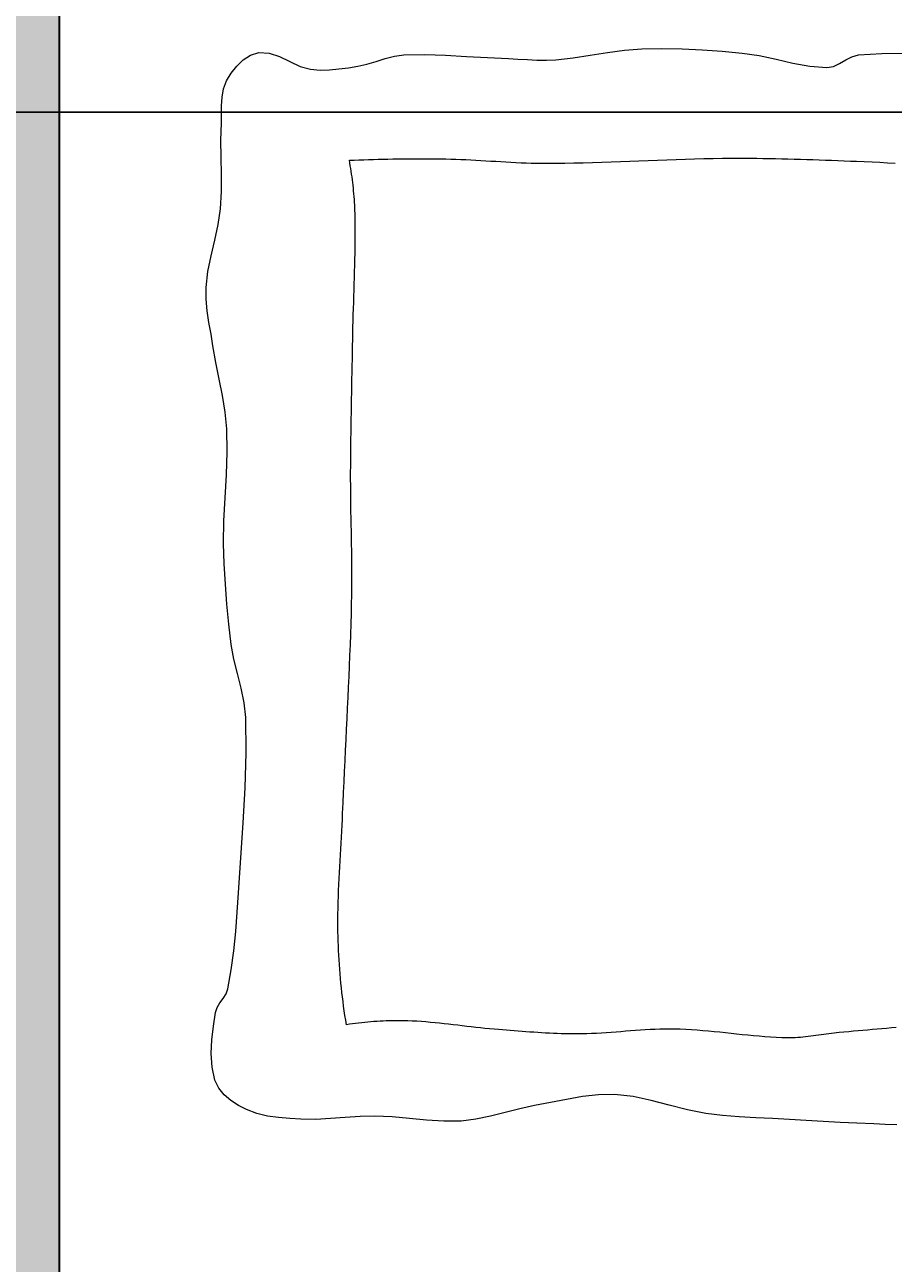
# Model space of a CAD drawing. Units: inches. Extents: x -15 to 423, y -713 to 71.
# Tile 11 of 24: x 251 to 308, y -351 to -270. Entities that reach past the tile are written whole.
import ezdxf

# ---------------------------------------------------------------- set-up
doc = ezdxf.new("R2010")
doc.units = ezdxf.units.IN
doc.header["$MEASUREMENT"] = 0
for name, color, linetype, lineweight in [('A-ANNO-DIMS', 2, 'Continuous', 18), ('A-FURN', 9, 'Continuous', 13), ('A-WALL', 7, 'Continuous', 35), ('A-WALL-PATT', 8, 'Continuous', 13)]:
    doc.layers.add(name, color=color, linetype=linetype, lineweight=lineweight)
doc.styles.get("Standard").update_dxf_attribs({"font": 'arial.ttf'})
doc.dimstyles.get("Standard").update_dxf_attribs({"dimtxt": 0.18, "dimasz": 0.18, "dimexe": 0.18, "dimexo": 0.0625, "dimgap": 0.09, "dimtad": 0, "dimtih": 1, "dimtoh": 1, "dimdec": 0, "dimzin": 0, "dimdsep": 46, "dimlunit": 3, "dimtxsty": 'Standard', "dimcen": 0.09, "dimadec": 0, "dimazin": 0, "dimtfac": 1, "dimtdec": 0, "dimtofl": 0, "dimtmove": 0, "dimatfit": 3, "dimfxl": 1, "dimtolj": 1, "dimtzin": 0, "dimarcsym": 0})

# ---------------------------------------------------------------- blocks, each defined once
blk = doc.blocks.new('BED-DOUBLE')
for p, q in [((2.003, 69.219), (2.429, 69.63)), ((2.429, 69.63), (2.912, 69.937)), ((2.912, 69.937), (3.444, 70.1)), ((3.444, 70.1), (4.136, 70.064)), ((4.136, 70.064), (4.809, 69.832)), ((4.809, 69.832), (5.474, 69.509)), ((11.118, 69.518), (11.713, 69.708)), ((11.713, 69.708), (12.313, 69.864)), ((12.313, 69.864), (12.925, 69.947)), ((12.925, 69.947), (14.291, 69.973)), ((14.291, 69.973), (15.658, 69.932)), ((15.658, 69.932), (17.025, 69.853)), ((17.025, 69.853), (18.393, 69.767)), ((18.393, 69.767), (19.76, 69.702)), ((19.76, 69.702), (20.382, 69.674)), ((20.382, 69.674), (21.004, 69.639)), ((21.004, 69.639), (21.626, 69.611)), ((21.626, 69.611), (22.247, 69.602)), ((22.247, 69.602), (22.868, 69.627)), ((22.868, 69.627), (23.993, 69.748)), ((23.993, 69.748), (25.114, 69.92)), ((25.114, 69.92), (26.233, 70.103)), ((26.233, 70.103), (27.355, 70.258)), ((27.355, 70.258), (28.482, 70.345)), ((28.482, 70.345), (29.796, 70.368)), ((29.796, 70.368), (31.11, 70.346)), ((31.11, 70.346), (32.424, 70.284)), ((32.424, 70.284), (33.736, 70.19)), ((33.736, 70.19), (35.045, 70.069)), ((35.045, 70.069), (36.156, 69.9)), ((36.156, 69.9), (37.259, 69.661)), ((37.259, 69.661), (38.359, 69.412)), ((41.413, 69.382), (41.81, 69.617)), ((41.81, 69.617), (42.214, 69.827)), ((42.214, 69.827), (42.641, 69.942)), ((42.641, 69.942), (44.16, 70.042)), ((44.16, 70.042), (45.684, 70.067)), ((1.638, 68.744), (2.003, 69.219)), ((5.474, 69.509), (6.146, 69.198)), ((6.146, 69.198), (6.838, 69.007)), ((6.838, 69.007), (7.451, 68.958)), ((7.451, 68.958), (8.068, 68.97)), ((8.068, 68.97), (8.686, 69.026)), ((8.686, 69.026), (9.302, 69.109)), ((9.302, 69.109), (9.914, 69.204)), ((9.914, 69.204), (10.52, 69.337)), ((10.52, 69.337), (11.118, 69.518)), ((38.359, 69.412), (39.464, 69.211)), ((39.464, 69.211), (40.58, 69.118)), ((40.58, 69.118), (41.008, 69.192)), ((41.008, 69.192), (41.413, 69.382)), ((1.142, 67.735), (1.339, 68.246)), ((1.339, 68.246), (1.638, 68.744)), ((1.014, 66.627), (1.045, 67.191)), ((1.045, 67.191), (1.142, 67.735)), ((1.011, 66.057), (1.014, 66.627)), ((1, 65.495), (1.011, 66.057)), ((0.976, 64.376), (1, 65.495)), ((0.991, 63.255), (0.976, 64.376)), ((1.011, 62.135), (0.991, 63.255)), ((10.94, 63.119), (11.255, 63.127)), ((11.255, 63.127), (11.57, 63.134)), ((11.57, 63.134), (11.885, 63.14)), ((11.885, 63.14), (12.2, 63.145)), ((12.2, 63.145), (12.515, 63.15)), ((12.515, 63.15), (12.83, 63.153)), ((12.83, 63.153), (13.145, 63.156)), ((13.145, 63.156), (13.46, 63.158)), ((13.46, 63.158), (13.775, 63.159)), ((13.775, 63.159), (14.09, 63.159)), ((14.09, 63.159), (14.405, 63.158)), ((14.405, 63.158), (14.72, 63.156)), ((14.72, 63.156), (15.035, 63.154)), ((15.035, 63.154), (15.35, 63.15)), ((15.35, 63.15), (15.665, 63.146)), ((15.665, 63.146), (15.993, 63.139)), ((15.993, 63.139), (16.321, 63.13)), ((16.321, 63.13), (16.649, 63.118)), ((30.721, 63.116), (31.328, 63.135)), ((31.328, 63.135), (31.935, 63.153)), ((31.935, 63.153), (32.542, 63.168)), ((32.542, 63.168), (33.148, 63.181)), ((33.148, 63.181), (33.755, 63.19)), ((33.755, 63.19), (34.362, 63.196)), ((34.362, 63.196), (34.77, 63.197)), ((34.77, 63.197), (35.178, 63.197)), ((35.178, 63.197), (35.586, 63.195)), ((35.586, 63.195), (35.994, 63.192)), ((35.994, 63.192), (36.402, 63.187)), ((36.402, 63.187), (36.81, 63.18)), ((36.81, 63.18), (37.218, 63.172)), ((37.218, 63.172), (37.626, 63.163)), ((37.626, 63.163), (38.034, 63.153)), ((38.034, 63.153), (38.442, 63.142)), ((38.442, 63.142), (38.85, 63.13)), ((38.85, 63.13), (39.258, 63.117)), ((9.366, 63.066), (9.681, 63.078)), ((9.399, 62.885), (9.366, 63.066)), ((9.431, 62.703), (9.399, 62.885)), ((9.461, 62.522), (9.431, 62.703)), ((9.49, 62.34), (9.461, 62.522)), ((9.518, 62.157), (9.49, 62.34)), ((9.681, 63.078), (9.995, 63.09)), ((9.995, 63.09), (10.31, 63.1)), ((10.31, 63.1), (10.625, 63.11)), ((10.625, 63.11), (10.94, 63.119)), ((16.649, 63.118), (16.978, 63.104)), ((16.978, 63.104), (17.306, 63.088)), ((17.306, 63.088), (17.634, 63.07)), ((17.634, 63.07), (17.962, 63.052)), ((17.962, 63.052), (18.29, 63.032)), ((18.29, 63.032), (18.618, 63.013)), ((18.618, 63.013), (18.946, 62.993)), ((18.946, 62.993), (19.274, 62.973)), ((19.274, 62.973), (19.602, 62.954)), ((19.602, 62.954), (19.93, 62.937)), ((19.93, 62.937), (20.258, 62.92)), ((20.258, 62.92), (20.586, 62.905)), ((20.586, 62.905), (20.914, 62.893)), ((20.914, 62.893), (21.242, 62.882)), ((21.242, 62.882), (21.57, 62.875)), ((21.57, 62.875), (21.899, 62.87)), ((21.899, 62.87), (22.227, 62.869)), ((22.227, 62.869), (22.834, 62.873)), ((22.834, 62.873), (23.441, 62.88)), ((23.441, 62.88), (24.048, 62.891)), ((24.048, 62.891), (24.654, 62.905)), ((24.654, 62.905), (25.261, 62.921)), ((25.261, 62.921), (25.868, 62.94)), ((25.868, 62.94), (26.475, 62.96)), ((26.475, 62.96), (27.081, 62.982)), ((27.081, 62.982), (27.688, 63.004)), ((27.688, 63.004), (28.295, 63.027)), ((28.295, 63.027), (28.901, 63.05)), ((28.901, 63.05), (29.508, 63.073)), ((29.508, 63.073), (30.115, 63.095)), ((30.115, 63.095), (30.721, 63.116)), ((39.258, 63.117), (39.666, 63.103)), ((39.666, 63.103), (40.073, 63.089)), ((40.073, 63.089), (40.481, 63.074)), ((40.481, 63.074), (40.889, 63.059)), ((40.889, 63.059), (41.297, 63.044)), ((41.297, 63.044), (41.705, 63.028)), ((41.705, 63.028), (42.112, 63.013)), ((42.112, 63.013), (42.52, 62.997)), ((42.52, 62.997), (43.024, 62.977)), ((43.024, 62.977), (43.528, 62.954)), ((43.528, 62.954), (44.032, 62.93)), ((44.032, 62.93), (44.535, 62.904)), ((44.535, 62.904), (45.039, 62.877)), ((1.006, 61.015), (1.011, 62.135)), ((9.543, 61.975), (9.518, 62.157)), ((9.568, 61.792), (9.543, 61.975)), ((9.59, 61.609), (9.568, 61.792)), ((9.612, 61.426), (9.59, 61.609)), ((0.942, 59.899), (1.006, 61.015)), ((9.631, 61.242), (9.612, 61.426)), ((9.649, 61.059), (9.631, 61.242)), ((9.666, 60.875), (9.649, 61.059)), ((9.681, 60.691), (9.666, 60.875)), ((0.791, 58.864), (0.942, 59.899)), ((9.694, 60.507), (9.681, 60.691)), ((9.706, 60.323), (9.694, 60.507)), ((9.717, 60.139), (9.706, 60.323)), ((9.726, 59.955), (9.717, 60.139)), ((9.733, 59.771), (9.726, 59.955)), ((9.739, 59.587), (9.733, 59.771)), ((9.743, 59.403), (9.739, 59.587)), ((9.749, 59.001), (9.743, 59.403)), ((0.568, 57.839), (0.791, 58.864)), ((9.752, 58.599), (9.749, 59.001)), ((9.753, 58.197), (9.752, 58.599)), ((0.326, 56.816), (0.568, 57.839)), ((9.746, 57.392), (9.751, 57.794)), ((9.751, 57.794), (9.753, 58.197)), ((0.119, 55.79), (0.326, 56.816)), ((9.732, 56.588), (9.74, 56.99)), ((9.74, 56.99), (9.746, 57.392)), ((9.713, 55.784), (9.723, 56.186)), ((9.723, 56.186), (9.732, 56.588)), ((0, 54.752), (0.119, 55.79)), ((9.689, 54.98), (9.701, 55.382)), ((9.701, 55.382), (9.713, 55.784)), ((0.002, 53.985), (0, 54.752)), ((9.663, 54.176), (9.676, 54.578)), ((9.676, 54.578), (9.689, 54.98)), ((0.074, 53.22), (0.002, 53.985)), ((9.637, 53.371), (9.65, 53.773)), ((9.65, 53.773), (9.663, 54.176)), ((0.191, 52.456), (0.074, 53.22)), ((9.614, 52.567), (9.625, 52.969)), ((9.625, 52.969), (9.637, 53.371)), ((0.325, 51.694), (0.191, 52.456)), ((9.594, 51.763), (9.603, 52.165)), ((9.603, 52.165), (9.614, 52.567)), ((0.451, 50.932), (0.325, 51.694)), ((9.579, 50.926), (9.586, 51.361)), ((9.586, 51.361), (9.594, 51.763)), ((0.64, 49.847), (0.451, 50.932)), ((9.562, 50.055), (9.571, 50.49)), ((9.571, 50.49), (9.579, 50.926)), ((0.862, 48.766), (0.64, 49.847)), ((9.546, 49.185), (9.554, 49.62)), ((9.554, 49.62), (9.562, 50.055)), ((1.08, 47.685), (0.862, 48.766)), ((9.529, 48.315), (9.537, 48.75)), ((9.537, 48.75), (9.546, 49.185)), ((9.512, 47.444), (9.521, 47.879)), ((9.521, 47.879), (9.529, 48.315)), ((1.261, 46.6), (1.08, 47.685)), ((9.497, 46.574), (9.505, 47.009)), ((9.505, 47.009), (9.512, 47.444)), ((1.369, 45.507), (1.261, 46.6)), ((9.483, 45.704), (9.49, 46.139)), ((9.49, 46.139), (9.497, 46.574)), ((1.392, 44.009), (1.369, 45.507)), ((9.477, 45.268), (9.483, 45.704)), ((9.466, 44.398), (9.471, 44.833)), ((9.471, 44.833), (9.477, 45.268)), ((1.334, 42.51), (1.392, 44.009)), ((9.457, 43.528), (9.461, 43.963)), ((9.461, 43.963), (9.466, 44.398)), ((9.452, 42.657), (9.454, 43.092)), ((9.454, 43.092), (9.457, 43.528)), ((1.242, 41.01), (1.334, 42.51)), ((9.451, 42.232), (9.452, 42.657)), ((9.453, 41.806), (9.451, 42.232)), ((9.456, 41.38), (9.453, 41.806)), ((9.461, 40.954), (9.456, 41.38)), ((1.164, 39.51), (1.242, 41.01)), ((9.467, 40.529), (9.461, 40.954)), ((9.474, 40.103), (9.467, 40.529)), ((9.481, 39.677), (9.474, 40.103)), ((9.489, 39.251), (9.481, 39.677)), ((1.147, 38.01), (1.164, 39.51)), ((9.497, 38.826), (9.489, 39.251)), ((9.505, 38.4), (9.497, 38.826)), ((9.513, 37.974), (9.505, 38.4)), ((1.189, 36.691), (1.147, 38.01)), ((9.519, 37.548), (9.513, 37.974)), ((9.525, 37.123), (9.519, 37.548)), ((1.262, 35.372), (1.189, 36.691)), ((9.53, 36.697), (9.525, 37.123)), ((9.533, 36.271), (9.53, 36.697)), ((9.535, 35.846), (9.533, 36.271)), ((9.534, 35.42), (9.535, 35.846)), ((1.364, 34.055), (1.262, 35.372)), ((9.525, 34.569), (9.531, 34.994)), ((9.531, 34.994), (9.534, 35.42)), ((1.493, 32.741), (1.364, 34.055)), ((9.499, 33.455), (9.517, 34.143)), ((9.517, 34.143), (9.525, 34.569)), ((9.479, 32.766), (9.499, 33.455)), ((1.648, 31.429), (1.493, 32.741)), ((9.457, 32.078), (9.479, 32.766)), ((9.433, 31.389), (9.457, 32.078)), ((1.821, 30.468), (1.648, 31.429)), ((9.406, 30.701), (9.433, 31.389)), ((2.058, 29.516), (1.821, 30.468)), ((9.349, 29.324), (9.378, 30.012)), ((9.378, 30.012), (9.406, 30.701)), ((2.303, 28.566), (2.058, 29.516)), ((9.318, 28.636), (9.349, 29.324)), ((2.502, 27.612), (2.303, 28.566)), ((9.286, 27.948), (9.318, 28.636)), ((2.6, 26.645), (2.502, 27.612)), ((9.254, 27.26), (9.286, 27.948)), ((9.221, 26.572), (9.254, 27.26)), ((2.618, 24.352), (2.6, 26.645)), ((9.187, 25.883), (9.221, 26.572)), ((9.12, 24.507), (9.153, 25.195)), ((9.153, 25.195), (9.187, 25.883)), ((2.555, 22.06), (2.618, 24.352)), ((9.086, 23.819), (9.12, 24.507)), ((9.053, 23.131), (9.086, 23.819)), ((9.02, 22.443), (9.053, 23.131)), ((2.435, 19.769), (2.555, 22.06)), ((8.989, 21.755), (9.02, 22.443)), ((8.929, 20.378), (8.958, 21.066)), ((8.958, 21.066), (8.989, 21.755)), ((8.912, 19.992), (8.929, 20.378)), ((2.283, 17.478), (2.435, 19.769)), ((8.873, 19.219), (8.893, 19.606)), ((8.893, 19.606), (8.912, 19.992)), ((8.83, 18.447), (8.852, 18.833)), ((8.852, 18.833), (8.873, 19.219)), ((8.785, 17.674), (8.807, 18.06)), ((8.807, 18.06), (8.83, 18.447)), ((2.127, 15.19), (2.283, 17.478)), ((8.74, 16.901), (8.762, 17.288)), ((8.762, 17.288), (8.785, 17.674)), ((8.699, 16.129), (8.719, 16.515)), ((8.719, 16.515), (8.74, 16.901)), ((8.664, 15.356), (8.681, 15.742)), ((8.681, 15.742), (8.699, 16.129)), ((2.039, 13.928), (2.127, 15.19)), ((8.628, 14.197), (8.637, 14.583)), ((8.637, 14.583), (8.649, 14.97)), ((8.649, 14.97), (8.664, 15.356)), ((1.937, 12.667), (2.039, 13.928)), ((8.619, 13.424), (8.622, 13.81)), ((8.622, 13.81), (8.628, 14.197)), ((8.619, 13.037), (8.619, 13.424)), ((8.624, 12.651), (8.619, 13.037)), ((1.808, 11.408), (1.937, 12.667)), ((8.631, 12.346), (8.624, 12.651)), ((8.64, 12.04), (8.631, 12.346)), ((1.642, 10.155), (1.808, 11.408)), ((8.651, 11.735), (8.64, 12.04)), ((8.664, 11.43), (8.651, 11.735)), ((8.679, 11.125), (8.664, 11.43)), ((8.697, 10.82), (8.679, 11.125)), ((8.717, 10.516), (8.697, 10.82)), ((1.43, 8.91), (1.642, 10.155)), ((8.739, 10.211), (8.717, 10.516)), ((8.763, 9.906), (8.739, 10.211)), ((8.79, 9.602), (8.763, 9.906)), ((1.31, 8.587), (1.43, 8.91)), ((8.818, 9.298), (8.79, 9.602)), ((8.849, 8.994), (8.818, 9.298)), ((8.883, 8.69), (8.849, 8.994)), ((0.905, 7.999), (1.119, 8.289)), ((1.119, 8.289), (1.31, 8.587)), ((8.918, 8.387), (8.883, 8.69)), ((8.955, 8.084), (8.918, 8.387)), ((0.489, 6.488), (0.615, 7.375)), ((0.615, 7.375), (0.72, 7.7)), ((0.72, 7.7), (0.905, 7.999)), ((8.995, 7.781), (8.955, 8.084)), ((9.037, 7.479), (8.995, 7.781)), ((9.081, 7.176), (9.037, 7.479)), ((0.386, 5.589), (0.489, 6.488)), ((9.127, 6.875), (9.081, 7.176)), ((9.176, 6.573), (9.127, 6.875)), ((9.374, 6.604), (9.176, 6.573)), ((9.573, 6.633), (9.374, 6.604)), ((9.773, 6.66), (9.573, 6.633)), ((9.972, 6.685), (9.773, 6.66)), ((10.172, 6.708), (9.972, 6.685)), ((10.372, 6.729), (10.172, 6.708)), ((10.573, 6.748), (10.372, 6.729)), ((10.773, 6.766), (10.573, 6.748)), ((10.974, 6.781), (10.773, 6.766)), ((11.175, 6.795), (10.974, 6.781)), ((11.376, 6.806), (11.175, 6.795)), ((11.577, 6.816), (11.376, 6.806)), ((11.778, 6.824), (11.577, 6.816)), ((11.979, 6.83), (11.778, 6.824)), ((12.18, 6.834), (11.979, 6.83)), ((12.382, 6.836), (12.18, 6.834)), ((12.583, 6.836), (12.382, 6.836)), ((12.784, 6.835), (12.583, 6.836)), ((12.985, 6.831), (12.784, 6.835)), ((13.186, 6.826), (12.985, 6.831)), ((13.483, 6.814), (13.186, 6.826)), ((13.781, 6.798), (13.483, 6.814)), ((14.078, 6.779), (13.781, 6.798)), ((14.375, 6.756), (14.078, 6.779)), ((14.672, 6.731), (14.375, 6.756)), ((14.969, 6.703), (14.672, 6.731)), ((15.265, 6.673), (14.969, 6.703)), ((15.561, 6.641), (15.265, 6.673)), ((15.858, 6.607), (15.561, 6.641)), ((16.154, 6.573), (15.858, 6.607)), ((16.45, 6.538), (16.154, 6.573)), ((16.746, 6.503), (16.45, 6.538)), ((17.043, 6.467), (16.746, 6.503)), ((17.339, 6.432), (17.043, 6.467)), ((17.635, 6.398), (17.339, 6.432)), ((17.932, 6.366), (17.635, 6.398)), ((18.228, 6.334), (17.932, 6.366)), ((18.525, 6.305), (18.228, 6.334)), ((18.822, 6.278), (18.525, 6.305)), ((19.119, 6.254), (18.822, 6.278)), ((19.375, 6.234), (19.119, 6.254)), ((19.63, 6.214), (19.375, 6.234)), ((19.886, 6.194), (19.63, 6.214)), ((20.142, 6.174), (19.886, 6.194)), ((20.398, 6.154), (20.142, 6.174)), ((20.654, 6.134), (20.398, 6.154)), ((20.91, 6.115), (20.654, 6.134)), ((21.166, 6.097), (20.91, 6.115)), ((21.423, 6.079), (21.166, 6.097)), ((21.679, 6.062), (21.423, 6.079)), ((21.935, 6.047), (21.679, 6.062)), ((22.191, 6.032), (21.935, 6.047)), ((22.448, 6.019), (22.191, 6.032)), ((22.704, 6.007), (22.448, 6.019)), ((22.96, 5.997), (22.704, 6.007)), ((23.217, 5.988), (22.96, 5.997)), ((23.473, 5.981), (23.217, 5.988)), ((23.73, 5.977), (23.473, 5.981)), ((23.986, 5.974), (23.73, 5.977)), ((24.243, 5.973), (23.986, 5.974)), ((24.562, 5.977), (24.243, 5.973)), ((24.881, 5.985), (24.562, 5.977)), ((25.201, 5.996), (24.881, 5.985)), ((25.52, 6.012), (25.201, 5.996)), ((25.839, 6.03), (25.52, 6.012)), ((26.158, 6.051), (25.839, 6.03)), ((26.477, 6.073), (26.158, 6.051)), ((26.796, 6.097), (26.477, 6.073)), ((27.115, 6.121), (26.796, 6.097)), ((27.434, 6.146), (27.115, 6.121)), ((27.753, 6.17), (27.434, 6.146)), ((28.072, 6.194), (27.753, 6.17)), ((28.391, 6.216), (28.072, 6.194)), ((28.71, 6.236), (28.391, 6.216)), ((29.029, 6.253), (28.71, 6.236)), ((29.348, 6.268), (29.029, 6.253)), ((29.667, 6.279), (29.348, 6.268)), ((29.986, 6.286), (29.667, 6.279)), ((30.305, 6.288), (29.986, 6.286)), ((30.625, 6.284), (30.305, 6.288)), ((30.994, 6.274), (30.625, 6.284)), ((31.364, 6.259), (30.994, 6.274)), ((31.732, 6.238), (31.364, 6.259)), ((32.101, 6.213), (31.732, 6.238)), ((32.47, 6.183), (32.101, 6.213)), ((32.838, 6.151), (32.47, 6.183)), ((33.206, 6.116), (32.838, 6.151)), ((33.574, 6.079), (33.206, 6.116)), ((33.943, 6.041), (33.574, 6.079)), ((34.311, 6.002), (33.943, 6.041)), ((34.679, 5.963), (34.311, 6.002)), ((35.047, 5.925), (34.679, 5.963)), ((35.415, 5.888), (35.047, 5.925)), ((35.783, 5.853), (35.415, 5.888)), ((36.152, 5.82), (35.783, 5.853)), ((36.52, 5.791), (36.152, 5.82)), ((36.889, 5.765), (36.52, 5.791)), ((37.258, 5.743), (36.889, 5.765)), ((37.627, 5.727), (37.258, 5.743)), ((37.996, 5.716), (37.627, 5.727)), ((38.167, 5.715), (37.996, 5.716)), ((38.337, 5.717), (38.167, 5.715)), ((38.507, 5.724), (38.337, 5.717)), ((38.676, 5.733), (38.507, 5.724)), ((38.846, 5.746), (38.676, 5.733)), ((39.016, 5.761), (38.846, 5.746)), ((39.185, 5.779), (39.016, 5.761)), ((39.354, 5.798), (39.185, 5.779)), ((39.524, 5.82), (39.354, 5.798)), ((39.693, 5.842), (39.524, 5.82)), ((39.862, 5.865), (39.693, 5.842)), ((40.031, 5.889), (39.862, 5.865)), ((40.201, 5.914), (40.031, 5.889)), ((40.37, 5.938), (40.201, 5.914)), ((40.539, 5.961), (40.37, 5.938)), ((40.708, 5.984), (40.539, 5.961)), ((40.878, 6.006), (40.708, 5.984)), ((41.047, 6.026), (40.878, 6.006)), ((41.217, 6.045), (41.047, 6.026)), ((41.386, 6.061), (41.217, 6.045)), ((41.696, 6.089), (41.386, 6.061)), ((42.005, 6.117), (41.696, 6.089)), ((42.315, 6.145), (42.005, 6.117)), ((42.624, 6.173), (42.315, 6.145)), ((42.934, 6.201), (42.624, 6.173)), ((43.243, 6.229), (42.934, 6.201)), ((43.552, 6.257), (43.243, 6.229)), ((43.862, 6.284), (43.552, 6.257)), ((44.171, 6.312), (43.862, 6.284)), ((44.481, 6.338), (44.171, 6.312)), ((44.791, 6.365), (44.481, 6.338)), ((45.1, 6.391), (44.791, 6.365)), ((0.342, 4.691), (0.386, 5.589)), ((0.396, 3.805), (0.342, 4.691)), ((0.585, 2.944), (0.396, 3.805)), ((0.826, 2.44), (0.585, 2.944)), ((1.185, 1.996), (0.826, 2.44)), ((1.628, 1.613), (1.185, 1.996)), ((23.558, 1.698), (22.516, 1.488)), ((24.602, 1.881), (23.558, 1.698)), ((25.65, 2), (24.602, 1.881)), ((26.702, 2.017), (25.65, 2)), ((27.907, 1.881), (26.702, 2.017)), ((29.096, 1.626), (27.907, 1.881)), ((30.278, 1.316), (29.096, 1.626)), ((2.124, 1.291), (1.628, 1.613)), ((2.637, 1.029), (2.124, 1.291)), ((3.313, 0.777), (2.637, 1.029)), ((19.558, 0.843), (18.603, 0.6)), ((20.513, 1.087), (19.558, 0.843)), ((21.476, 1.289), (20.513, 1.087)), ((22.516, 1.488), (21.476, 1.289)), ((31.462, 1.013), (30.278, 1.316)), ((32.658, 0.783), (31.462, 1.013)), ((4.018, 0.609), (3.313, 0.777)), ((4.74, 0.502), (4.018, 0.609)), ((5.471, 0.439), (4.74, 0.502)), ((6.198, 0.398), (5.471, 0.439)), ((7.166, 0.391), (6.198, 0.398)), ((8.135, 0.443), (7.166, 0.391)), ((9.104, 0.52), (8.135, 0.443)), ((10.073, 0.587), (9.104, 0.52)), ((11.042, 0.61), (10.073, 0.587)), ((12.169, 0.556), (11.042, 0.61)), ((13.295, 0.449), (12.169, 0.556)), ((14.42, 0.337), (13.295, 0.449)), ((15.545, 0.264), (14.42, 0.337)), ((16.67, 0.279), (15.545, 0.264)), ((17.642, 0.398), (16.67, 0.279)), ((18.603, 0.6), (17.642, 0.398)), ((33.747, 0.653), (32.658, 0.783)), ((34.84, 0.562), (33.747, 0.653)), ((35.936, 0.496), (34.84, 0.562)), ((37.033, 0.44), (35.936, 0.496)), ((38.129, 0.378), (37.033, 0.44)), ((39.231, 0.31), (38.129, 0.378)), ((40.333, 0.246), (39.231, 0.31)), ((41.435, 0.186), (40.333, 0.246)), ((42.538, 0.134), (41.435, 0.186)), ((43.641, 0.088), (42.538, 0.134)), ((44.395, 0.056), (43.641, 0.088)), ((45.149, 0.023), (44.395, 0.056))]:
    blk.add_line(p, q)
blk = doc.blocks.new('*D38')
at = {"layer": 'A-ANNO-DIMS', "color": 0, "lineweight": -2, "transparency": 16777216}
for p, q in [((124.143, -240.5), (422.011, -240.5)), ((421.831, -240.68), (421.831, -258.055)), ((421.831, -275.796), (421.831, -258.421)), ((124.143, -275.976), (422.011, -275.976))]:
    blk.add_line(p, q, dxfattribs=at)
at = {"layer": 'A-ANNO-DIMS', "color": 0, "transparency": 16777216}
for points in [[(421.801, -240.68), (421.861, -240.68), (421.831, -240.5)], [(421.801, -275.796), (421.861, -275.796), (421.831, -275.976)]]:
    blk.add_solid(points, dxfattribs=at)
at = {"layer": 'Defpoints', "color": 0, "transparency": 16777216}
for p in [(124.081, -240.5), (124.081, -275.976), (421.831, -275.976)]:
    blk.add_point(p, dxfattribs=at)
at = {"layer": 'A-ANNO-DIMS', "color": 0, "transparency": 16777216, "insert": (421.831, -258.238), "char_height": 0.18, "attachment_point": 5}
blk.add_mtext('\\A1;2\'-11 1/2"', dxfattribs=at)

msp = doc.modelspace()

# ---------------------------------------------------------------- hatches: boundary and pattern name
at = {"layer": 'A-WALL-PATT'}
h = msp.add_hatch(color=256, dxfattribs=at)
h.dxf.hatch_style = 1
h.paths.add_polyline_path([(34.081, -349.58), (25.081, -349.58), (25.081, -431), (34.081, -431)])
h.paths.add_polyline_path([(34.081, -467), (25.081, -467), (25.081, -673), (34.081, -673)])
h.paths.add_polyline_path([(373.081, -668.5), (182.081, -668.5), (182.081, -673), (373.081, -673)])
h.paths.add_polyline_path([(253.199, -597.5), (191.081, -597.5), (191.081, -594.5), (182.081, -594.5), (182.081, -606.5), (253.199, -606.5)])
h.paths.add_polyline_path([(373.081, -597.5), (313.199, -597.5), (313.199, -606.5), (373.081, -606.5)])
h.paths.add_polyline_path([(382.081, -545.549), (373.081, -545.549), (373.081, -673), (382.081, -673)])
h.paths.add_polyline_path([(139.081, -488), (34.081, -488), (34.081, -497), (139.081, -497), (139.081, -492.5)])
h.paths.add_polyline_path([(139.081, -396.5), (128.581, -396.5), (128.581, -352.79), (124.081, -352.79), (124.081, -396.5), (34.081, -396.5), (34.081, -410), (139.081, -410), (139.081, -403.25)])
h.paths.add_polyline_path([(191.081, -396.5), (179.081, -396.5), (179.081, -410), (182.081, -410), (182.081, -488), (179.081, -488), (179.081, -497), (182.081, -497), (182.081, -501.431), (191.081, -501.431)])
h.paths.add_polyline_path([(373.081, -396.5), (253.081, -396.5), (253.081, -393.5), (248.581, -393.5), (248.581, -401), (284.581, -401), (284.581, -404), (289.081, -404), (289.081, -401), (373.081, -401)])
h.paths.add_polyline_path([(373.081, -449), (289.081, -449), (289.081, -432), (286.831, -432), (284.581, -432), (284.581, -453.5), (373.081, -453.5)])
h.paths.add_polyline_path([(382.081, -344.267), (373.081, -344.267), (373.081, -413.683), (382.081, -413.683)])
h.paths.add_polyline_path([(382.081, -437.683), (373.081, -437.683), (373.081, -485.549), (382.081, -485.549)])
h.paths.add_polyline_path([(34.081, -188.264), (25.081, -188.264), (25.081, -289.58), (34.081, -289.58)])
h.paths.add_polyline_path([(164.081, -236), (34.081, -236), (34.081, -240.5), (124.081, -240.5), (124.081, -293.122), (128.581, -293.122), (128.581, -240.5), (164.081, -240.5), (164.081, -238.25)])
h.paths.add_polyline_path([(373.081, -236), (242.581, -236), (242.581, -238.25), (242.581, -240.5), (248.581, -240.5), (248.581, -353.5), (250.831, -353.5), (253.081, -353.5), (253.081, -240.5), (373.081, -240.5)])
h.paths.add_polyline_path([(382.081, -190.86), (373.081, -190.86), (373.081, -284.267), (382.081, -284.267)])
h.paths.add_polyline_path([(211.581, -80), (253.581, -80), (253.581, -77.75), (253.581, -75.5), (153.581, -75.5), (153.581, -77.75), (153.581, -80), (207.081, -80), (207.081, -236), (204.081, -236), (204.081, -240.5), (214.581, -240.5), (214.581, -236), (211.581, -236)])
h.paths.add_polyline_path([(34.081, 8.5), (70.358, 8.5), (70.358, 17.5), (25.081, 17.5), (25.081, -128.264), (34.081, -128.264)])
h.paths.add_polyline_path([(110.581, 17.5), (94.358, 17.5), (94.358, 8.5), (110.581, 8.5)])
h.paths.add_polyline_path([(296.581, 17.5), (110.581, 17.5), (110.581, 13), (296.581, 13)])
h.paths.add_polyline_path([(110.581, 8.5), (106.081, 8.5), (106.081, -75.5), (103.081, -75.5), (103.081, -80), (113.581, -80), (113.581, -77.75), (113.581, -75.5), (110.581, -75.5)])
h.paths.add_polyline_path([(75.081, -75.5), (34.081, -75.5), (34.081, -80), (75.081, -80), (75.081, -77.75)])
h.paths.add_polyline_path([(343.093, 17.5), (296.581, 17.5), (296.581, 13), (296.581, 8.5), (343.093, 8.5)])
h.paths.add_polyline_path([(304.081, -75.5), (301.081, -75.5), (301.081, 8.5), (296.581, 8.5), (296.581, -75.5), (293.581, -75.5), (293.581, -80), (304.081, -80)])
h.paths.add_polyline_path([(382.081, 17.5), (367.093, 17.5), (367.093, 8.5), (373.081, 8.5), (373.081, -130.86), (382.081, -130.86)])
h.paths.add_polyline_path([(373.081, -75.5), (332.081, -75.5), (332.081, -77.75), (332.081, -80), (373.081, -80)])

# ---------------------------------------------------------------- linework, layer by layer
at = {"layer": 'A-WALL'}
msp.add_line((253.081, -240.5), (253.081, -353.5), dxfattribs=at)

# ---------------------------------------------------------------- block references
at = {"layer": 'A-FURN'}
msp.add_blockref('BED-DOUBLE', (262.678, -342.175), dxfattribs=at)

# ---------------------------------------------------------------- dimensions: what is measured, and where the dimension line sits
at = {"layer": 'A-ANNO-DIMS'}
dim = msp.add_linear_dim(base=(421.831, -275.976), p1=(124.081, -240.5), p2=(124.081, -275.976), angle=90, dimstyle='Standard', override={"dimdec": 1, "dimlfac": 1, "dimrnd": 0, "dimzin": 1, "dimdsep": 46, "dimlunit": 4, "dimfrac": 2}, dxfattribs=at)
dim.commit()
dim.dimension.update_dxf_attribs({"geometry": '*D38', "text_midpoint": (421.831, -258.238)})

doc.saveas('drawing.dxf')
